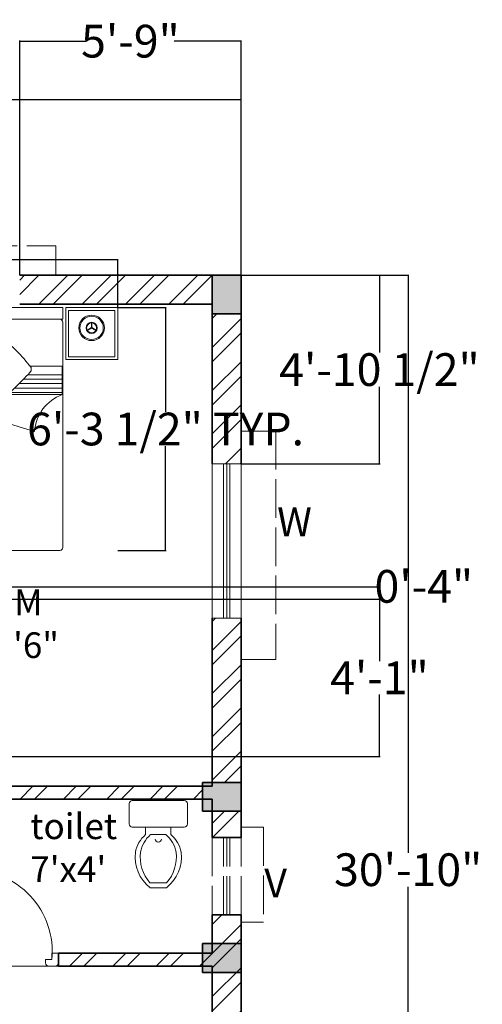
# Model space of a CAD drawing. Units: inches. Extents: x 2379 to 3013, y 1431 to 2110.
# Tile 10 of 10: x 2869 to 3013, y 1795 to 2101. Entities that reach past the tile are written whole.
import ezdxf

# ---------------------------------------------------------------- set-up
doc = ezdxf.new("R2010")
doc.units = ezdxf.units.IN
doc.linetypes.add('ACAD_ISO02W100', pattern=[15, 12, -3])
for name, color, linetype, lineweight in [('00 FURNITURE', 15, 'Continuous', 15), ('A-ANNO-DIMS', 2, 'Continuous', 18), ('A-ANNO-TEXT', 7, 'Continuous', 18), ('A-AREA-IDEN', 7, 'Continuous', 18), ('A-COLS', 7, 'Continuous', 35), ('A-COLS-PATT', 252, 'Continuous', 13), ('A-DOOR', 4, 'Continuous', 18), ('A-FLOR-FIXT', 9, 'Continuous', 18), ('A-GLAZ-VENT', 6, 'ACAD_ISO02W100', 13), ('A-ROOF-OVHD', 11, 'ACAD_ISO02W100', 13), ('A-WALL-PATT', 8, 'Continuous', 13), ('A_FUR 1', 5, 'Continuous', 5), ('WALL', 7, 'Continuous', 35), ('WINDOW', 4, 'Continuous', 15)]:
    doc.layers.add(name, color=color, linetype=linetype, lineweight=lineweight)
doc.styles.get("Standard").update_dxf_attribs({"font": 'arial.ttf'})
doc.dimstyles.get("Standard").update_dxf_attribs({"dimtxt": 10.18, "dimasz": 0.18, "dimexe": 0.18, "dimexo": 0.0625, "dimgap": 0.09, "dimtad": 0, "dimtih": 1, "dimtoh": 1, "dimdec": 0, "dimzin": 0, "dimdsep": 46, "dimlunit": 3, "dimtxsty": 'Standard', "dimcen": 0.09, "dimadec": 0, "dimazin": 0, "dimtfac": 1, "dimtdec": 0, "dimtofl": 0, "dimtmove": 0, "dimatfit": 3, "dimfxl": 1, "dimtolj": 1, "dimtzin": 0, "dimarcsym": 0})

# ---------------------------------------------------------------- blocks, each defined once
blk = doc.blocks.new('column')
for p, q in [((2588.21, 2021.79), (2597.21, 2021.79)), ((2588.21, 2009.79), (2588.21, 2021.79)), ((2597.21, 2021.79), (2597.21, 2009.79)), ((2597.21, 2009.79), (2588.21, 2009.79))]:
    blk.add_line(p, q)
blk = doc.blocks.new('ESTSET')
at = {"layer": 'A_FUR 1'}
for p, q in [((-10.44, 4.1), (-10.44, 32.1)), ((-8.44, 4.1), (-8.44, 32.1)), ((-36.44, 6.1), (-36.44, 3.1)), ((-34.44, 6.1), (-36.44, 6.1)), ((-34.44, 4.1), (-34.44, 6.1)), ((-34.44, 4.1), (-34.44, 6.1)), ((-32.44, 4.1), (-34.44, 4.1)), ((-32.44, 4.1), (-34.44, 4.1)), ((-32.44, 3.1), (-32.44, 4.1)), ((-10.44, 3.1), (-10.44, 4.1)), ((-10.44, 4.1), (-8.44, 4.1)), ((-10.44, 4.1), (-8.44, 4.1)), ((-8.44, 4.1), (-8.44, 6.1)), ((-8.44, 6.1), (-6.44, 6.1)), ((-8.44, 4.1), (-8.44, 6.1)), ((-6.44, 6.1), (-6.44, 3.1)), ((-6.44, 2.1), (-36.44, 2.1)), ((-35.44, 2.1), (-33.44, 2.1)), ((-7.44, 2.1), (-9.44, 2.1))]:
    blk.add_line(p, q, dxfattribs=at)
for points in [[(-21.44, 2.1), (-18.67, 2.1), (-18.67, 5.1), (-20.06, 5.1)], [(-20.06, 5.1), (-20.06, -0.91)], [(-21.44, 2.1), (-21.44, -0.91), (-20.06, -0.91)]]:
    blk.add_lwpolyline(points, dxfattribs=at)
for centre, radius, start, end in [((-8.91, 6.46), 25.64, 88.9606, 185.2816), ((-35.44, 3.1), 1, 180, 270), ((-33.44, 3.1), 1, 270, 0), ((-9.44, 3.1), 1, 180, 270), ((-7.44, 3.1), 1, 270, 0)]:
    blk.add_arc(centre, radius, start, end, dxfattribs=at)
blk = doc.blocks.new('RGWTG')
at = {"layer": '00 FURNITURE'}
for p, q in [((578.23, 3473.51), (577.36, 3475.01)), ((578.36, 3473.58), (577.49, 3475.09)), ((578.23, 3473.58), (577.36, 3472.08)), ((578.36, 3473.51), (577.49, 3472)), ((578.29, 3473.62), (580.03, 3473.62)), ((578.29, 3473.47), (580.03, 3473.47)), ((521.93, 3464.58), (509.03, 3451.68)), ((509.03, 3422.63), (509.03, 3463.68)), ((509.93, 3464.58), (566.4, 3464.58)), ((557.53, 3463.84), (557.53, 3464.49)), ((557.53, 3464.49), (566.4, 3464.49)), ((558.2, 3464.49), (558.2, 3435.82)), ((559.57, 3464.49), (559.57, 3437.25)), ((560.94, 3464.49), (560.94, 3438.58)), ((562.3, 3464.49), (562.3, 3439.83)), ((563.67, 3464.49), (563.67, 3440.99)), ((565.04, 3464.49), (565.04, 3442.08)), ((566.4, 3464.58), (580.98, 3464.58)), ((566.4, 3464.49), (566.4, 3442.08)), ((566.4, 3464.49), (566.4, 3463.84)), ((580.98, 3464.58), (580.98, 3416.72)), ((558.2, 3426.48), (558.2, 3425.04)), ((509.03, 3400.68), (509.03, 3422.63)), ((580.98, 3416.72), (580.98, 3400.68)), ((558.2, 3416.13), (558.2, 3399.95)), ((559.57, 3414.75), (559.57, 3399.95)), ((560.94, 3413.39), (560.94, 3399.95)), ((562.3, 3412.04), (562.3, 3399.95)), ((563.67, 3410.72), (563.67, 3399.95)), ((580.08, 3399.78), (509.93, 3399.78)), ((557.53, 3399.95), (557.53, 3400.6)), ((566.4, 3399.95), (557.53, 3399.95)), ((566.4, 3400.6), (566.4, 3399.95)), ((578.23, 3390.78), (577.36, 3392.29)), ((578.36, 3390.86), (577.49, 3392.36)), ((578.23, 3390.86), (577.36, 3389.36)), ((578.36, 3390.78), (577.49, 3389.28)), ((578.29, 3390.9), (580.03, 3390.9)), ((578.29, 3390.74), (580.03, 3390.74))]:
    blk.add_line(p, q, dxfattribs=at)
for points in [[(568.43, 3465.48), (584.63, 3465.48), (584.63, 3481.68), (568.43, 3481.68)], [(569.33, 3466.38), (583.73, 3466.38), (583.73, 3480.78), (569.33, 3480.78)], [(580.98, 3399.78), (584.63, 3399.78), (584.63, 3464.58), (580.98, 3464.58)], [(568.43, 3398.88), (584.63, 3398.88), (584.63, 3382.68), (568.43, 3382.68)], [(569.33, 3397.98), (583.73, 3397.98), (583.73, 3383.58), (569.33, 3383.58)]]:
    blk.add_lwpolyline(points, close=True, dxfattribs=at)
for points in [[(566.52, 3464.49), (557.53, 3464.49), (557.53, 3435.08)], [(557.53, 3427.21), (557.53, 3424.3)], [(557.53, 3416.82), (557.53, 3399.95), (566.4, 3399.95), (566.4, 3409.94)]]:
    blk.add_lwpolyline(points, dxfattribs=at)
for centre, radius in [((578.29, 3473.54), 3.97), ((578.29, 3473.54), 3.63), ((578.29, 3473.54), 1.74), ((578.29, 3473.54), 1.56), ((578.29, 3390.82), 3.97), ((578.29, 3390.82), 3.63), ((578.29, 3390.82), 1.74), ((578.29, 3390.82), 1.56)]:
    blk.add_circle(centre, radius, dxfattribs=at)
for centre, radius, start, end in [((509.93, 3463.68), 0.9, 90, 180), ((529.65, 3456.88), 10.9, 135.0361, 191.9278), ((290.56, 3490.52), 268.3, 342.2214, 354.2925), ((516.73, 3443.97), 10.9, 78.0722, 134.9639), ((598.15, 3399.01), 54.32, 127.931, 142.069), ((566.05, 3440.57), 1.82, 45, 135), ((533.58, 3399.31), 54.32, 37.931, 52.069), ((556.59, 3431.11), 1.82, 135, 225), ((574.84, 3431.77), 1.82, 315, 45), ((597.87, 3463.6), 54.32, 217.931, 224.141), ((598.15, 3388.23), 54.32, 127.931, 142.069), ((566.05, 3429.78), 1.82, 45, 135), ((533.58, 3388.53), 54.32, 37.931, 52.069), ((533.28, 3463.88), 54.32, 316.32, 322.069), ((556.59, 3420.33), 1.82, 135, 225), ((533.28, 3453.1), 54.32, 307.931, 322.069), ((574.84, 3420.99), 1.82, 315, 45), ((765.33, 3619.75), 290.45, 223.6069, 226.2326), ((545.02, 3395.29), 13.35, 20.4224, 85.5825), ((565.44, 3411.05), 1.47, 225.9674, 326.8337), ((509.93, 3400.68), 0.9, 180, 270), ((580.08, 3400.68), 0.9, 270, 0)]:
    blk.add_arc(centre, radius, start, end, dxfattribs=at)
blk = doc.blocks.new('A$C2AC94788')
for p, q in [((0, 0.505), (0, 0.665)), ((0.025, 0.69), (0.435, 0.69)), ((0.46, 0.665), (0.46, 0.505)), ((0.435, 0.48), (0.025, 0.48)), ((0.13, 0.48), (0.13, 0.42)), ((0.33, 0.42), (0.33, 0.48)), ((0.17, 0.42), (0.29, 0.42)), ((0.1641, 0.0392), (0.2959, 0.0392)), ((0.2291, 0.0392), (0.23, 0.0392)), ((0.2309, 0.0392), (0.23, 0.0392)), ((0.165, 0), (0.295, 0))]:
    blk.add_line(p, q)
for centre, radius, start, end in [((0.025, 0.665), 0.025, 90, 180), ((0.435, 0.665), 0.025, 0, 90), ((0.025, 0.505), 0.025, 180, 270), ((0.435, 0.505), 0.025, 270, 0), ((0.2874, 0.2356), 0.2425, 130.48854, 169.44501), ((0.3274, 0.2356), 0.2425, 130.48854, 169.44501), ((0.1326, 0.2356), 0.2425, 10.55499, 49.51146), ((0.1726, 0.2356), 0.2425, 10.55499, 49.51146), ((0.23, 0.385), 0.025, 180, 0), ((0.3601, 0.2448), 0.313, 173.53688, 231.44828), ((0.4001, 0.2448), 0.313, 173.53688, 221.06038), ((0.0999, 0.2448), 0.313, 308.55172, 6.46312), ((0.0599, 0.2448), 0.313, 318.93962, 6.46312)]:
    blk.add_arc(centre, radius, start, end)
blk = doc.blocks.new('*D14')
at = {"layer": 'A-ANNO-DIMS', "color": 0, "lineweight": -2, "transparency": 16777216}
for p, q in [((2469.63, 2021.67), (2469.63, 2076.34)), ((2469.81, 2076.16), (2694.9, 2076.16)), ((2937.45, 2076.16), (2712.35, 2076.16)), ((2937.63, 2021.67), (2937.63, 2076.34))]:
    blk.add_line(p, q, dxfattribs=at)
at = {"layer": 'A-ANNO-DIMS', "color": 0, "transparency": 16777216}
for points in [[(2469.81, 2076.19), (2469.81, 2076.13), (2469.63, 2076.16)], [(2937.45, 2076.19), (2937.45, 2076.13), (2937.63, 2076.16)]]:
    blk.add_solid(points, dxfattribs=at)
at = {"layer": 'Defpoints', "color": 0, "transparency": 16777216}
for p in [(2937.63, 2076.16), (2469.63, 2021.61), (2937.63, 2021.61)]:
    blk.add_point(p, dxfattribs=at)
at = {"layer": 'A-ANNO-DIMS', "color": 0, "transparency": 16777216, "insert": (2703.63, 2076.16), "char_height": 10.18, "attachment_point": 5}
blk.add_mtext("\\A1;39'", dxfattribs=at)
blk = doc.blocks.new('*D15')
at = {"layer": 'A-ANNO-DIMS', "color": 0, "lineweight": -2, "transparency": 16777216}
for p, q in [((2937.69, 2021.61), (2989.73, 2021.61)), ((2989.55, 2021.43), (2989.55, 1841.9)), ((2989.55, 1651.79), (2989.55, 1831.32)), ((2937.69, 1651.61), (2989.73, 1651.61))]:
    blk.add_line(p, q, dxfattribs=at)
at = {"layer": 'A-ANNO-DIMS', "color": 0, "transparency": 16777216}
for points in [[(2989.52, 2021.43), (2989.58, 2021.43), (2989.55, 2021.61)], [(2989.52, 1651.79), (2989.58, 1651.79), (2989.55, 1651.61)]]:
    blk.add_solid(points, dxfattribs=at)
at = {"layer": 'Defpoints', "color": 0, "transparency": 16777216}
for p in [(2937.63, 2021.61), (2937.62, 1651.61), (2989.55, 1651.61)]:
    blk.add_point(p, dxfattribs=at)
at = {"layer": 'A-ANNO-DIMS', "color": 0, "transparency": 16777216, "insert": (2989.55, 1836.61), "char_height": 10.18, "attachment_point": 5}
blk.add_mtext('\\A1;30\'-10"', dxfattribs=at)
blk = doc.blocks.new('WIN-48IN')
for p, q in [((0, 48), (0, 0)), ((9, 48), (0, 48)), ((3.5, 48), (3.5, 0)), ((4.5, 48), (4.5, 0)), ((5.5, 48), (5.5, 0)), ((9, 0), (9, 48)), ((9, 0), (0, 0))]:
    blk.add_line(p, q)
blk = doc.blocks.new('VENT-24IN')
for p, q in [((24, 5.5), (0, 5.5)), ((24, 4.5), (0, 4.5)), ((24, 3.5), (0, 3.5))]:
    blk.add_line(p, q)
blk.add_lwpolyline([(0, 9), (0, 0), (24, 0), (24, 9)], close=True)
blk = doc.blocks.new('*D30')
at = {"layer": 'A-ANNO-DIMS', "color": 0, "lineweight": -2, "transparency": 16777216}
for p, q in [((2800.26, 2026.41), (2800.08, 2026.41)), ((2800.26, 2011.63), (2800.26, 2026.59)), ((2899.08, 2026.41), (2800.44, 2026.41)), ((2899.26, 2011.63), (2899.26, 2026.59))]:
    blk.add_line(p, q, dxfattribs=at)
at = {"layer": 'A-ANNO-DIMS', "color": 0, "transparency": 16777216}
for points in [[(2800.44, 2026.44), (2800.44, 2026.38), (2800.26, 2026.41)], [(2899.08, 2026.44), (2899.08, 2026.38), (2899.26, 2026.41)]]:
    blk.add_solid(points, dxfattribs=at)
at = {"layer": 'Defpoints', "color": 0, "transparency": 16777216}
for p in [(2800.26, 2026.41), (2800.26, 2011.56), (2899.26, 2011.56)]:
    blk.add_point(p, dxfattribs=at)
at = {"layer": 'A-ANNO-DIMS', "color": 0, "transparency": 16777216, "insert": (2724.54, 2026.41), "char_height": 10.18, "attachment_point": 5}
blk.add_mtext('\\A1;BED GROUP 8\'-3" TYP.', dxfattribs=at)
blk = doc.blocks.new('*D31')
at = {"layer": 'A-ANNO-DIMS', "color": 0, "lineweight": -2, "transparency": 16777216}
for p, q in [((2899.32, 2011.56), (2914.29, 2011.56)), ((2914.11, 2011.38), (2914.11, 1979.12)), ((2914.11, 1936.14), (2914.11, 1968.41)), ((2899.32, 1935.96), (2914.29, 1935.96))]:
    blk.add_line(p, q, dxfattribs=at)
at = {"layer": 'A-ANNO-DIMS', "color": 0, "transparency": 16777216}
for points in [[(2914.08, 2011.38), (2914.14, 2011.38), (2914.11, 2011.56)], [(2914.08, 1936.14), (2914.14, 1936.14), (2914.11, 1935.96)]]:
    blk.add_solid(points, dxfattribs=at)
at = {"layer": 'Defpoints', "color": 0, "transparency": 16777216}
for p in [(2899.26, 2011.56), (2914.11, 2011.56), (2899.26, 1935.96)]:
    blk.add_point(p, dxfattribs=at)
at = {"layer": 'A-ANNO-DIMS', "color": 0, "transparency": 16777216, "insert": (2914.11, 1973.76), "char_height": 10.18, "attachment_point": 5}
blk.add_mtext('\\A1;6\'-3 1/2" TYP.', dxfattribs=at)
blk = doc.blocks.new('*D54')
at = {"layer": 'A-ANNO-DIMS', "color": 0, "lineweight": -2, "transparency": 16777216}
for p, q in [((2735.39, 1920.79), (2980.8, 1920.79)), ((2980.62, 1920.61), (2980.62, 1901.53)), ((2980.62, 1872.05), (2980.62, 1891.13)), ((2735.39, 1871.87), (2980.8, 1871.87))]:
    blk.add_line(p, q, dxfattribs=at)
at = {"layer": 'A-ANNO-DIMS', "color": 0, "transparency": 16777216}
for points in [[(2980.59, 1920.61), (2980.65, 1920.61), (2980.62, 1920.79)], [(2980.59, 1872.05), (2980.65, 1872.05), (2980.62, 1871.87)]]:
    blk.add_solid(points, dxfattribs=at)
at = {"layer": 'Defpoints', "color": 0, "transparency": 16777216}
for p in [(2735.32, 1920.79), (2980.62, 1920.79), (2735.32, 1871.87)]:
    blk.add_point(p, dxfattribs=at)
at = {"layer": 'A-ANNO-DIMS', "color": 0, "transparency": 16777216, "insert": (2980.62, 1896.33), "char_height": 10.18, "attachment_point": 5}
blk.add_mtext('\\A1;4\'-1"', dxfattribs=at)
blk = doc.blocks.new('*D60')
at = {"layer": 'A-ANNO-DIMS', "color": 0, "lineweight": -2, "transparency": 16777216}
for p, q in [((2868.76, 2021.67), (2868.76, 2094.64)), ((2868.94, 2094.46), (2889.57, 2094.46)), ((2937.45, 2094.46), (2916.81, 2094.46)), ((2937.63, 2021.67), (2937.63, 2094.64))]:
    blk.add_line(p, q, dxfattribs=at)
at = {"layer": 'A-ANNO-DIMS', "color": 0, "transparency": 16777216}
for points in [[(2868.94, 2094.49), (2868.94, 2094.43), (2868.76, 2094.46)], [(2937.45, 2094.49), (2937.45, 2094.43), (2937.63, 2094.46)]]:
    blk.add_solid(points, dxfattribs=at)
at = {"layer": 'Defpoints', "color": 0, "transparency": 16777216}
for p in [(2937.63, 2094.46), (2868.76, 2021.61), (2937.63, 2021.61)]:
    blk.add_point(p, dxfattribs=at)
at = {"layer": 'A-ANNO-DIMS', "color": 0, "transparency": 16777216, "insert": (2903.19, 2094.46), "char_height": 10.18, "attachment_point": 5}
blk.add_mtext('\\A1;5\'-9"', dxfattribs=at)
blk = doc.blocks.new('*D61')
at = {"layer": 'A-ANNO-DIMS', "color": 0, "lineweight": -2, "transparency": 16777216}
for p, q in [((2937.69, 2021.61), (2980.8, 2021.61)), ((2980.62, 2021.43), (2980.62, 1997.61)), ((2980.62, 1963.08), (2980.62, 1986.9)), ((2937.69, 1962.9), (2980.8, 1962.9))]:
    blk.add_line(p, q, dxfattribs=at)
at = {"layer": 'A-ANNO-DIMS', "color": 0, "transparency": 16777216}
for points in [[(2980.59, 2021.43), (2980.65, 2021.43), (2980.62, 2021.61)], [(2980.59, 1963.08), (2980.65, 1963.08), (2980.62, 1962.9)]]:
    blk.add_solid(points, dxfattribs=at)
at = {"layer": 'Defpoints', "color": 0, "transparency": 16777216}
for p in [(2937.63, 2021.61), (2980.62, 2021.61), (2937.63, 1962.9)]:
    blk.add_point(p, dxfattribs=at)
at = {"layer": 'A-ANNO-DIMS', "color": 0, "transparency": 16777216, "insert": (2980.62, 1992.25), "char_height": 10.18, "attachment_point": 5}
blk.add_mtext('\\A1;4\'-10 1/2"', dxfattribs=at)
blk = doc.blocks.new('*D66')
at = {"layer": 'A-ANNO-DIMS', "color": 0, "lineweight": -2, "transparency": 16777216}
for p, q in [((2763.69, 1924.61), (2980.8, 1924.61)), ((2980.62, 1924.61), (2980.62, 1924.79)), ((2980.62, 1924.79), (2980.8, 1924.79)), ((2980.62, 1920.97), (2980.62, 1924.43)), ((2735.39, 1920.79), (2980.8, 1920.79))]:
    blk.add_line(p, q, dxfattribs=at)
at = {"layer": 'A-ANNO-DIMS', "color": 0, "transparency": 16777216}
for points in [[(2980.59, 1924.43), (2980.65, 1924.43), (2980.62, 1924.61)], [(2980.59, 1920.97), (2980.65, 1920.97), (2980.62, 1920.79)]]:
    blk.add_solid(points, dxfattribs=at)
at = {"layer": 'Defpoints', "color": 0, "transparency": 16777216}
for p in [(2763.63, 1924.61), (2980.62, 1924.61), (2735.32, 1920.79)]:
    blk.add_point(p, dxfattribs=at)
at = {"layer": 'A-ANNO-DIMS', "color": 0, "transparency": 16777216, "insert": (2994.42, 1924.79), "char_height": 10.18, "attachment_point": 5}
blk.add_mtext('\\A1;0\'-4"', dxfattribs=at)

msp = doc.modelspace()

# ---------------------------------------------------------------- hatches: boundary and pattern name
at = {"layer": 'A-COLS-PATT'}
h = msp.add_hatch(color=256, dxfattribs=at)
h.dxf.hatch_style = 1
h.paths.add_polyline_path([(2937.62, 1660.61), (2925.62, 1660.61), (2925.62, 1651.61), (2937.62, 1651.61)])
h.paths.add_polyline_path([(2481.63, 1809.61), (2478.63, 1809.61), (2478.63, 1811.02), (2469.63, 1811.02), (2469.63, 1802.02), (2478.63, 1802.02), (2478.63, 1805.61), (2481.63, 1805.61)])
h.paths.add_polyline_path([(2481.63, 1811.02), (2478.63, 1811.02), (2478.63, 1809.61), (2481.63, 1809.61)], flags=17)
h.paths.add_polyline_path([(2481.63, 1805.61), (2478.63, 1805.61), (2478.63, 1802.02), (2481.63, 1802.02)], flags=17)
h.paths.add_polyline_path([(2481.63, 1660.61), (2469.63, 1660.61), (2469.63, 1651.61), (2481.63, 1651.61)])
h.paths.add_polyline_path([(2692.07, 1660.61), (2688.63, 1660.61), (2688.63, 1663.61), (2684.63, 1663.61), (2684.63, 1660.61), (2683.07, 1660.61), (2683.07, 1651.61), (2692.07, 1651.61)])
h.paths.add_polyline_path([(2692.07, 1663.61), (2688.63, 1663.61), (2688.63, 1660.61), (2692.07, 1660.61)], flags=17)
h.paths.add_polyline_path([(2684.63, 1663.61), (2683.07, 1663.61), (2683.07, 1660.61), (2684.63, 1660.61)], flags=17)
h.paths.add_polyline_path([(2770.63, 1660.61), (2767.63, 1660.61), (2767.63, 1663.61), (2763.63, 1663.61), (2763.63, 1660.61), (2761.63, 1660.61), (2761.63, 1651.61), (2763.63, 1651.61), (2767.63, 1651.61), (2767.63, 1651.61), (2770.63, 1651.61)])
h.paths.add_polyline_path([(2770.63, 1663.61), (2767.63, 1663.61), (2767.63, 1660.61), (2770.63, 1660.61)], flags=17)
h.paths.add_polyline_path([(2763.63, 1663.61), (2761.63, 1663.61), (2761.63, 1660.61), (2763.63, 1660.61)], flags=17)
h.paths.add_polyline_path([(2937.63, 1813.62), (2928.63, 1813.62), (2928.63, 1810.61), (2925.63, 1810.61), (2925.63, 1806.61), (2928.63, 1806.61), (2928.63, 1804.62), (2937.63, 1804.62)], flags=17)
h.paths.add_polyline_path([(2937.63, 1813.62), (2928.63, 1813.62), (2928.63, 1810.61), (2925.63, 1810.61), (2925.63, 1804.62), (2937.63, 1804.62)], flags=17)
h.paths.add_polyline_path([(2928.63, 1813.62), (2925.63, 1813.62), (2925.63, 1810.61), (2928.63, 1810.61)], flags=0)
h.paths.add_polyline_path([(2937.63, 1863.8), (2928.63, 1863.8), (2928.63, 1862.61), (2925.63, 1862.61), (2925.63, 1858.61), (2928.63, 1858.61), (2928.63, 1854.8), (2937.63, 1854.8)])
h.paths.add_polyline_path([(2928.63, 1863.8), (2925.63, 1863.8), (2925.63, 1862.61), (2928.63, 1862.61)], flags=17)
h.paths.add_polyline_path([(2928.63, 1858.61), (2925.63, 1858.61), (2925.63, 1854.8), (2928.63, 1854.8)], flags=17)
h.paths.add_polyline_path([(2937.63, 2021.61), (2928.63, 2021.61), (2928.63, 2012.61), (2928.63, 2012.61), (2928.63, 2009.61), (2937.63, 2009.61)])
h.paths.add_polyline_path([(2770.27, 2021.61), (2761.27, 2021.61), (2761.27, 2012.61), (2763.63, 2012.61), (2763.63, 2009.61), (2767.63, 2009.61), (2767.63, 2012.61), (2770.27, 2012.61)])
h.paths.add_polyline_path([(2763.63, 2012.61), (2761.27, 2012.61), (2761.27, 2009.61), (2763.63, 2009.61)], flags=17)
h.paths.add_polyline_path([(2770.27, 2012.61), (2767.63, 2012.61), (2767.63, 2009.61), (2770.27, 2009.61)], flags=17)
h.paths.add_polyline_path([(2597.21, 2021.61), (2588.21, 2021.61), (2588.21, 2012.61), (2590.63, 2012.61), (2590.63, 2009.61), (2594.63, 2009.61), (2594.63, 2012.61), (2597.21, 2012.61)])
h.paths.add_polyline_path([(2590.63, 2012.61), (2588.21, 2012.61), (2588.21, 2009.61), (2590.63, 2009.61)], flags=17)
h.paths.add_polyline_path([(2597.21, 2012.61), (2594.63, 2012.61), (2594.63, 2009.61), (2597.21, 2009.61)], flags=17)
h = msp.add_hatch(color=256, dxfattribs=at)
h.dxf.hatch_style = 1
h.paths.add_polyline_path([(2937.63, 1813.62), (2928.63, 1813.62), (2928.63, 1810.61), (2925.63, 1810.61), (2925.63, 1806.61), (2928.63, 1806.61), (2928.63, 1804.62), (2937.63, 1804.62)])
h.paths.add_polyline_path([(2928.63, 1813.62), (2925.63, 1813.62), (2925.63, 1810.61), (2928.63, 1810.61)], flags=17)
h.paths.add_polyline_path([(2693.63, 1810.71), (2684.63, 1810.71), (2684.63, 1810.61), (2688.63, 1810.61), (2688.63, 1798.71), (2693.63, 1798.71)])
h.paths.add_polyline_path([(2688.63, 1810.61), (2684.63, 1810.61), (2684.63, 1798.71), (2688.63, 1798.71)], flags=17)
h.paths.add_polyline_path([(2772.63, 1806.61), (2767.63, 1806.61), (2767.63, 1798.71), (2772.63, 1798.71)], flags=17)
h.paths.add_polyline_path([(2772.63, 1810.61), (2763.63, 1810.61), (2763.63, 1798.71), (2767.63, 1798.71), (2767.63, 1806.61), (2772.63, 1806.61)])
h.paths.add_polyline_path([(2773.54, 1858.61), (2763.63, 1858.61), (2763.63, 1862.61), (2761.54, 1862.61), (2761.54, 1853.61), (2773.54, 1853.61)])
h.paths.add_polyline_path([(2773.54, 1862.61), (2763.63, 1862.61), (2763.63, 1858.61), (2773.54, 1858.61)], flags=17)
h.paths.add_polyline_path([(2598.8, 1854.61), (2594.63, 1854.61), (2594.63, 1845.61), (2598.8, 1845.61)])
h.paths.add_polyline_path([(2594.63, 1854.61), (2590.63, 1854.61), (2590.63, 1845.61), (2594.63, 1845.61)])
h.paths.add_polyline_path([(2590.63, 1854.61), (2586.8, 1854.61), (2586.8, 1845.61), (2590.63, 1845.61)])
at = {"layer": 'A-WALL-PATT'}
h = msp.add_hatch(dxfattribs=at)
h.set_pattern_fill('ANSI32', color=256)
h.paths.add_polyline_path([(2925.63, 1862.61), (2815.63, 1862.61), (2815.63, 1858.61), (2827.63, 1858.61), (2827.63, 1810.61), (2815.63, 1810.61), (2815.63, 1806.61), (2850.78, 1806.61), (2850.78, 1810.61), (2831.63, 1810.61), (2831.63, 1858.61), (2925.63, 1858.61)])
h.paths.add_polyline_path([(2925.63, 1810.61), (2880.78, 1810.61), (2880.78, 1806.61), (2925.63, 1806.61)], flags=17)
h.paths.add_polyline_path([(2633.75, 1660.61), (2594.63, 1660.61), (2481.63, 1660.61), (2481.63, 1651.61), (2588.63, 1651.61), (2588.63, 1570.61), (2624.28, 1570.61), (2624.28, 1574.61), (2592.63, 1574.61), (2592.63, 1651.61), (2633.75, 1651.61)])
h.paths.add_polyline_path([(2594.63, 1809.61), (2481.63, 1809.61), (2481.63, 1805.61), (2594.63, 1805.61)])
h.paths.add_polyline_path([(2594.63, 2012.61), (2597.21, 2012.61), (2597.21, 2021.61), (2588.21, 2021.61), (2588.21, 2012.61), (2590.63, 2012.61), (2590.63, 1845.61), (2594.63, 1845.61)])
h.paths.add_polyline_path([(2767.63, 2012.61), (2770.27, 2012.61), (2770.27, 2021.61), (2761.27, 2021.61), (2761.27, 2012.61), (2763.63, 2012.61), (2763.63, 1928.61), (2691.63, 1928.61), (2643.63, 1928.61), (2643.63, 1924.61), (2691.63, 1924.61), (2763.63, 1924.61), (2763.63, 1858.61), (2779.63, 1858.61), (2779.63, 1862.61), (2767.63, 1862.61)])
h.paths.add_polyline_path([(2613.63, 2012.61), (2613.63, 2021.61), (2597.21, 2021.61), (2597.21, 2012.61)])
h.paths.add_polyline_path([(2508.33, 2012.61), (2508.33, 2021.61), (2478.63, 2021.61), (2478.63, 2012.61)])
h.paths.add_polyline_path([(2556.33, 2021.61), (2556.33, 2012.61), (2588.21, 2012.61), (2588.21, 2021.61)])
h.paths.add_polyline_path([(2659.15, 2012.61), (2659.15, 2021.61), (2643.63, 2021.61), (2643.63, 1958.61), (2661.63, 1958.61), (2661.63, 1962.61), (2647.63, 1962.61), (2647.63, 2012.61)])
h.paths.add_polyline_path([(2714.17, 2012.61), (2714.17, 2021.61), (2683.15, 2021.61), (2683.15, 2012.61), (2691.63, 2012.61), (2691.63, 1958.61), (2695.63, 1958.61), (2695.63, 2012.61)])
h.paths.add_polyline_path([(2738.17, 2021.61), (2738.17, 2012.61), (2761.27, 2012.61), (2761.27, 2021.61)])
h.paths.add_polyline_path([(2820.76, 2012.61), (2820.76, 2021.61), (2770.27, 2021.61), (2770.27, 2012.61)])
h.paths.add_polyline_path([(2868.76, 2021.61), (2868.76, 2012.61), (2928.63, 2012.61), (2928.63, 2021.61)])
h.paths.add_polyline_path([(2928.63, 1962.9), (2937.63, 1962.9), (2937.63, 2009.61), (2928.63, 2009.61)])
h.paths.add_polyline_path([(2937.63, 1914.9), (2928.63, 1914.9), (2928.63, 1863.8), (2937.63, 1863.8)])
h.paths.add_polyline_path([(2928.63, 1846.59), (2937.63, 1846.59), (2937.63, 1854.8), (2928.63, 1854.8)])
h.paths.add_polyline_path([(2937.63, 1822.59), (2928.63, 1822.59), (2928.63, 1813.62), (2937.63, 1813.62)])
h.paths.add_polyline_path([(2928.63, 1778.48), (2937.63, 1778.48), (2937.63, 1813.62), (2928.63, 1813.62), (2928.63, 1810.61), (2925.63, 1810.61), (2925.63, 1806.61), (2928.63, 1806.61)])
h.paths.add_polyline_path([(2816.22, 1651.61), (2816.22, 1660.61), (2767.63, 1660.61), (2767.63, 1806.61), (2779.63, 1806.61), (2779.63, 1810.61), (2763.63, 1810.61), (2763.63, 1660.61), (2688.63, 1660.61), (2688.63, 1810.61), (2684.63, 1810.61), (2684.63, 1660.61), (2669.75, 1660.61), (2669.75, 1651.61), (2763.63, 1651.61), (2763.63, 1574.61), (2672.28, 1574.61), (2672.28, 1570.61), (2767.63, 1570.61), (2767.63, 1651.61)])
h.paths.add_polyline_path([(2864.22, 1660.61), (2864.22, 1651.61), (2937.63, 1651.61), (2937.63, 1730.48), (2928.63, 1730.48), (2928.63, 1660.61)])
h.paths.add_polyline_path([(2469.63, 1975.19), (2478.63, 1975.19), (2478.63, 2009.61), (2469.63, 2009.61)])
h.paths.add_polyline_path([(2478.63, 1927.19), (2469.63, 1927.19), (2469.63, 1811.02), (2478.63, 1811.02)])
h.paths.add_polyline_path([(2469.63, 1758.04), (2478.63, 1758.04), (2478.63, 1802.02), (2469.63, 1802.02)])
h.paths.add_polyline_path([(2478.63, 1710.04), (2469.63, 1710.04), (2469.63, 1660.61), (2478.63, 1660.61)])

# ---------------------------------------------------------------- linework, layer by layer
at = {"layer": 'A-ROOF-OVHD'}
for p, q in [((2810.99, 2030.79), (2879.94, 2030.79)), ((2879.94, 2030.79), (2879.94, 2021.61)), ((2937.63, 1973.12), (2948.42, 1973.12)), ((2948.42, 1973.12), (2948.42, 1902.08)), ((2948.42, 1902.08), (2937.63, 1902.08)), ((2937.63, 1849.81), (2944.58, 1849.81)), ((2944.58, 1849.81), (2944.58, 1820.25)), ((2944.58, 1820.25), (2937.63, 1820.25))]:
    msp.add_line(p, q, dxfattribs=at)
at = {"layer": 'WALL'}
for p, q in [((2868.76, 2021.61), (2937.63, 2021.61)), ((2937.63, 2021.61), (2937.63, 1962.9)), ((2868.76, 2012.61), (2928.63, 2012.61)), ((2928.63, 2012.61), (2928.63, 1962.9)), ((2928.63, 1914.9), (2928.63, 1862.61)), ((2937.63, 1914.9), (2937.63, 1846.59)), ((2815.63, 1862.61), (2928.63, 1862.61)), ((2831.63, 1858.61), (2928.63, 1858.61)), ((2928.63, 1858.61), (2928.63, 1846.59)), ((2928.63, 1846.59), (2937.63, 1846.59)), ((2928.63, 1822.59), (2937.63, 1822.59)), ((2928.63, 1822.59), (2928.63, 1810.61)), ((2937.63, 1822.59), (2937.63, 1778.48)), ((2880.78, 1810.61), (2880.78, 1806.61)), ((2880.78, 1810.61), (2928.63, 1810.61)), ((2880.78, 1806.61), (2928.63, 1806.61)), ((2928.63, 1806.61), (2928.63, 1778.48))]:
    msp.add_line(p, q, dxfattribs=at)

# ---------------------------------------------------------------- block references
at = {"layer": '00 FURNITURE', "rotation": 89.99999999999999}
msp.add_blockref('RGWTG', (6281.94, 1426.94), dxfattribs=at)
at = {"layer": 'A-COLS'}
msp.add_blockref('column', (340.42, -0.18), dxfattribs=at)
at = {"layer": 'A-COLS', "rotation": 270}
for p in [(915.84, 4452.01), (915.84, 4401.83)]:
    msp.add_blockref('column', p, dxfattribs=at)
at = {"layer": 'A-DOOR', "xscale": -1}
msp.add_blockref('ESTSET', (2844.35, 1804.54), dxfattribs=at)
at = {"layer": 'A-FLOR-FIXT', "xscale": -39.375, "yscale": 39.375, "zscale": 39.375}
msp.add_blockref('A$C2AC94788', (2920.9, 1831), dxfattribs=at)
at = {"layer": 'A-GLAZ-VENT', "rotation": 269.9999999999949}
msp.add_blockref('VENT-24IN', (2928.63, 1846.59), dxfattribs=at)
at = {"layer": 'WINDOW', "rotation": 359.9999987925818}
msp.add_blockref('WIN-48IN', (2928.63, 1914.9), dxfattribs=at)

# ---------------------------------------------------------------- texts
at = {"layer": 'A-ANNO-TEXT', "char_height": 9, "attachment_point": 1}
for s, insert in [('W', (2948.81, 1949.36)), ('V', (2944.8, 1836.97))]:
    msp.add_mtext_dynamic_manual_height_columns(s, width=106.8919, gutter_width=12.5, heights=[0], dxfattribs=dict(at, insert=insert))
at = {"layer": 'A-AREA-IDEN', "char_height": 8, "attachment_point": 1}
for s, insert in [('BEDROOM                             13\'5"x12\'6"  ', (2822.77, 1923.82)), ("toilet\\P7'x4'        ", (2872.05, 1854.14))]:
    msp.add_mtext_dynamic_manual_height_columns(s, width=46.1506, gutter_width=12.5, heights=[0], dxfattribs=dict(at, insert=insert))

# ---------------------------------------------------------------- dimensions: what is measured, and where the dimension line sits
at = {"layer": 'A-ANNO-DIMS'}
for base, p1, override, picture, middle in [((2937.63, 2094.46), (2868.76, 2021.61), {"dimdec": 1, "dimlfac": 1, "dimrnd": 0, "dimzin": 1, "dimdsep": 46, "dimlunit": 4, "dimfrac": 2}, '*D60', (2903.19, 2094.46)), ((2937.63, 2076.16), (2469.63, 2021.61), {"dimclrd": 0, "dimclre": 0, "dimclrt": 0}, '*D14', (2703.63, 2076.16))]:
    dim = msp.add_linear_dim(base=base, p1=p1, p2=(2937.63, 2021.61), dimstyle='Standard', override=override, dxfattribs=at)
    dim.commit()
    dim.dimension.update_dxf_attribs({"geometry": picture, "text_midpoint": middle})
for base, p1, p2, angle, text, picture, middle in [((2800.26, 2026.41), (2899.26, 2011.56), (2800.26, 2011.56), 180, 'BED GROUP <> TYP.', '*D30', (2724.54, 2026.41)), ((2914.11, 2011.56), (2899.26, 1935.96), (2899.26, 2011.56), 90, '<> TYP.', '*D31', (2914.11, 1973.76))]:
    dim = msp.add_linear_dim(base=base, p1=p1, p2=p2, angle=angle, text=text, dimstyle='Standard', override={"dimdec": 1, "dimlfac": 1, "dimrnd": 0, "dimzin": 1, "dimdsep": 46, "dimlunit": 4, "dimfrac": 2}, dxfattribs=at)
    dim.commit()
    dim.dimension.update_dxf_attribs({"geometry": picture, "text_midpoint": middle})
for base, p1, p2, override, picture, middle in [((2989.55, 1651.61), (2937.63, 2021.61), (2937.62, 1651.61), {"dimclrd": 0, "dimclre": 0, "dimclrt": 0}, '*D15', (2989.55, 1836.61)), ((2980.62, 2021.61), (2937.63, 1962.9), (2937.63, 2021.61), {"dimdec": 1, "dimlfac": 1, "dimrnd": 0, "dimzin": 1, "dimdsep": 46, "dimlunit": 4, "dimfrac": 2}, '*D61', (2980.62, 1992.25)), ((2980.62, 1924.61), (2735.32, 1920.79), (2763.63, 1924.61), {"dimdec": 1, "dimlfac": 1, "dimrnd": 0, "dimzin": 1, "dimdsep": 46, "dimlunit": 4, "dimfrac": 2}, '*D66', (2994.42, 1924.79)), ((2980.62, 1920.79), (2735.32, 1871.87), (2735.32, 1920.79), {"dimdec": 1, "dimlfac": 1, "dimrnd": 0, "dimzin": 1, "dimdsep": 46, "dimlunit": 4, "dimfrac": 2}, '*D54', (2980.62, 1896.33))]:
    dim = msp.add_linear_dim(base=base, p1=p1, p2=p2, angle=90, dimstyle='Standard', override=override, dxfattribs=at)
    dim.commit()
    dim.dimension.update_dxf_attribs({"geometry": picture, "text_midpoint": middle})

doc.saveas('drawing.dxf')
